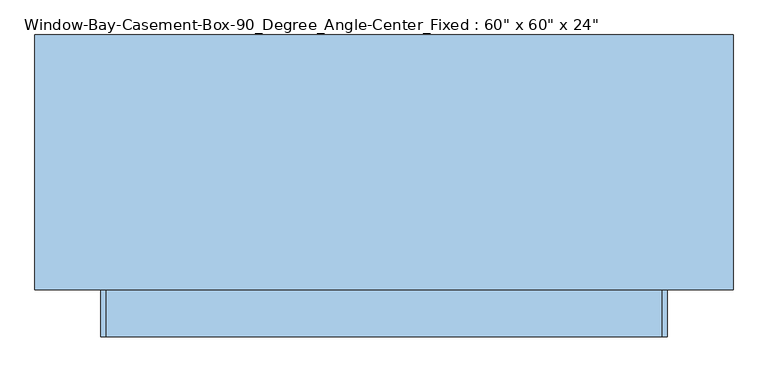
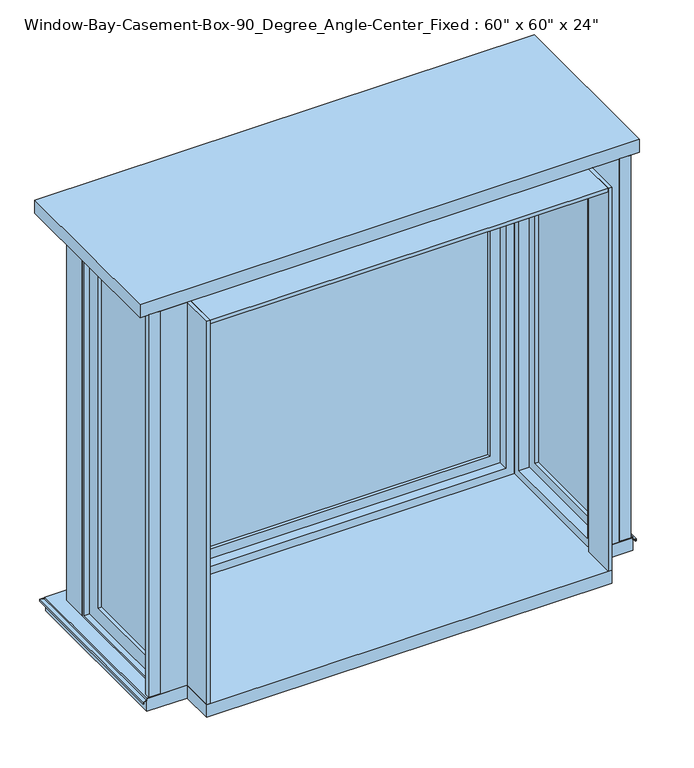
"""IFC4 building model written with IfcOpenShell, lengths in millimetres: window geometry."""

from ifc_helpers import new_model, si_unit, frame, origin, place, context, project, spatial, polyline, outline, extrude, faceted_brep, source, transform, mapped, element, save


def window_153fc52c(model_context):
    return source(origin(), model_context, "Body", "SolidModel", [
        extrude(outline(polyline([(-863.6, 63.5), (-908.05, 63.5), (-908.05, 82.55), (-863.6, 82.55), (-863.6, 63.5)])), frame((0.0, 0.0, 663.1486341), z_axis=(0.0, 0.0, 1.0), x_axis=(1.0, 0.0, 0.0)), (0.0, 0.0, 1.0), 1521.2513659),
        extrude(outline(polyline([(908.05, 63.5), (863.6, 63.5), (863.6, 82.55), (908.05, 82.55), (908.05, 63.5)])), frame((0.0, 0.0, 663.1486341), z_axis=(0.0, 0.0, 1.0), x_axis=(1.0, 0.0, 0.0)), (0.0, 0.0, 1.0), 1521.2513659),
        faceted_brep([(-914.4, 63.5, 653.0697935), (-914.4, 63.5, 660.4), (-863.6, 63.5, 660.4), (-863.6, 63.5, 663.1486341), (-915.797, 63.5, 663.1486341), (-915.797, 63.5, 654.4483503), (-928.497, 63.5, 652.2089977), (-928.497, 63.5, 643.2668038), (-924.5346, 63.5, 643.2668038), (-924.5346, 63.5, 644.7270038), (-926.8968, 63.5, 644.7270038), (-926.8968, 63.5, 650.8662705), (914.4, 63.5, 653.0697935), (926.8968, 63.5, 650.8662705), (926.8968, 63.5, 644.7270038), (924.5346, 63.5, 644.7270038), (924.5346, 63.5, 643.2668038), (928.497, 63.5, 643.2668038), (928.497, 63.5, 652.2089977), (915.797, 63.5, 654.4483503), (915.797, 63.5, 663.1486341), (863.6, 63.5, 663.1486341), (863.6, 63.5, 660.4), (914.4, 63.5, 660.4), (-914.4, 723.9, 653.0697935), (-914.4, 723.9, 660.4), (914.4, 723.9, 660.4), (863.6, 673.1, 660.4), (-863.6, 673.1, 660.4), (-863.6, 673.1, 663.1486341), (863.6, 673.1, 663.1486341), (915.797, 725.297, 663.1486341), (-915.797, 725.297, 663.1486341), (-915.797, 725.297, 654.4483503), (-928.497, 737.997, 652.2089977), (-928.497, 737.997, 643.2668038), (928.497, 737.997, 643.2668038), (924.5346, 734.0346, 643.2668038), (-924.5346, 734.0346, 643.2668038), (-924.5346, 734.0346, 644.7270038), (924.5346, 734.0346, 644.7270038), (926.8968, 736.3968, 644.7270038), (-926.8968, 736.3968, 644.7270038), (-926.8968, 736.3968, 650.8662705), (914.4, 723.9, 653.0697935), (915.797, 725.297, 654.4483503), (928.497, 737.997, 652.2089977), (926.8968, 736.3968, 650.8662705)], [[[0, 1, 2, 3, 4, 5, 6, 7, 8, 9, 10, 11]], [[12, 13, 14, 15, 16, 17, 18, 19, 20, 21, 22, 23]], [[1, 0, 24, 25]], [[2, 1, 25, 26, 23, 22, 27, 28]], [[3, 2, 28, 29]], [[4, 3, 29, 30, 21, 20, 31, 32]], [[5, 4, 32, 33]], [[6, 5, 33, 34]], [[7, 6, 34, 35]], [[8, 7, 35, 36, 17, 16, 37, 38]], [[9, 8, 38, 39]], [[10, 9, 39, 40, 15, 14, 41, 42]], [[11, 10, 42, 43]], [[0, 11, 43, 24]], [[25, 24, 44, 26]], [[29, 28, 27, 30]], [[33, 32, 31, 45]], [[34, 33, 45, 46]], [[35, 34, 46, 36]], [[39, 38, 37, 40]], [[43, 42, 41, 47]], [[24, 43, 47, 44]], [[26, 44, 12, 23]], [[30, 27, 22, 21]], [[45, 31, 20, 19]], [[46, 45, 19, 18]], [[36, 46, 18, 17]], [[40, 37, 16, 15]], [[47, 41, 14, 13]], [[44, 47, 13, 12]]]),
        extrude(outline(polyline([(914.4, 723.9), (914.4, 63.5), (762.0, 63.5), (762.0, -63.5), (-762.0, -63.5), (-762.0, 63.5), (-914.4, 63.5), (-914.4, 723.9), (914.4, 723.9)])), frame((0.0, 0.0, 609.6), z_axis=(0.0, 0.0, 1.0), x_axis=(1.0, 0.0, 0.0)), (0.0, 0.0, 1.0), 50.8),
        extrude(outline(polyline([(939.8, 749.3), (939.8, 63.5), (-939.8, 63.5), (-939.8, 749.3), (939.8, 749.3)])), frame((0.0, 0.0, 2184.4), z_axis=(0.0, 0.0, 1.0), x_axis=(1.0, 0.0, 0.0)), (0.0, 0.0, 1.0), 50.8),
        extrude(outline(polyline([(-762.0, 673.1), (-762.0, 571.5), (-863.6, 571.5), (-863.6, 673.1), (-762.0, 673.1)])), frame((0.0, 0.0, 660.4), z_axis=(0.0, 0.0, 1.0), x_axis=(1.0, 0.0, 0.0)), (0.0, 0.0, 1.0), 1524.0),
        extrude(outline(polyline([(863.6, 673.1), (863.6, 571.5), (762.0, 571.5), (762.0, 673.1), (863.6, 673.1)])), frame((0.0, 0.0, 660.4), z_axis=(0.0, 0.0, 1.0), x_axis=(1.0, 0.0, 0.0)), (0.0, 0.0, 1.0), 1524.0),
        faceted_brep([(749.3, 609.6, 673.1), (749.3, 673.1, 673.1), (-749.3, 673.1, 673.1), (-749.3, 609.6, 673.1), (730.25, 571.5, 692.15), (730.25, 609.6, 692.15), (-730.25, 609.6, 692.15), (-730.25, 571.5, 692.15), (762.0, 673.1, 660.4), (762.0, 571.5, 660.4), (-762.0, 571.5, 660.4), (-762.0, 673.1, 660.4), (-749.3, 673.1, 2171.7), (-749.3, 609.6, 2171.7), (-730.25, 609.6, 2152.65), (-730.25, 571.5, 2152.65), (-762.0, 571.5, 2184.4), (-762.0, 673.1, 2184.4), (749.3, 673.1, 2171.7), (749.3, 609.6, 2171.7), (730.25, 609.6, 2152.65), (730.25, 571.5, 2152.65), (762.0, 571.5, 2184.4), (762.0, 673.1, 2184.4)], [[[0, 1, 2, 3]], [[4, 5, 6, 7]], [[8, 9, 10, 11]], [[3, 2, 12, 13]], [[7, 6, 14, 15]], [[11, 10, 16, 17]], [[13, 12, 18, 19]], [[15, 14, 20, 21]], [[17, 16, 22, 23]], [[11, 17, 23, 8], [1, 18, 12, 2]], [[19, 18, 1, 0]], [[3, 13, 19, 0], [5, 20, 14, 6]], [[21, 20, 5, 4]], [[9, 22, 16, 10], [7, 15, 21, 4]], [[23, 22, 9, 8]]]),
        extrude(outline(polyline([(2171.7, -749.3), (673.1, -749.3), (673.1, 749.3), (2171.7, 749.3), (2171.7, -749.3)]), holes=[polyline([(2114.55, 692.15), (730.25, 692.15), (730.25, -692.15), (2114.55, -692.15), (2114.55, 692.15)])]), frame((0.0, 609.6, 0.0), z_axis=(0.0, 1.0, 0.0), x_axis=(0.0, 0.0, 1.0)), (0.0, 0.0, 1.0), 44.45),
        faceted_brep([(-762.0, 95.25, 2152.65), (-800.1, 95.25, 2152.65), (-800.1, 539.75, 2152.65), (-762.0, 539.75, 2152.65), (-863.6, 63.5, 2184.4), (-762.0, 63.5, 2184.4), (-762.0, 571.5, 2184.4), (-863.6, 571.5, 2184.4), (-800.1, 76.2, 2171.7), (-863.6, 76.2, 2171.7), (-863.6, 558.8, 2171.7), (-800.1, 558.8, 2171.7), (-800.1, 539.75, 692.15), (-762.0, 539.75, 692.15), (-762.0, 571.5, 660.4), (-863.6, 571.5, 660.4), (-863.6, 558.8, 673.1), (-800.1, 558.8, 673.1), (-800.1, 95.25, 692.15), (-762.0, 95.25, 692.15), (-762.0, 63.5, 660.4), (-863.6, 63.5, 660.4), (-863.6, 76.2, 673.1), (-800.1, 76.2, 673.1)], [[[0, 1, 2, 3]], [[4, 5, 6, 7]], [[8, 9, 10, 11]], [[3, 2, 12, 13]], [[7, 6, 14, 15]], [[11, 10, 16, 17]], [[13, 12, 18, 19]], [[15, 14, 20, 21]], [[17, 16, 22, 23]], [[11, 17, 23, 8], [1, 18, 12, 2]], [[19, 18, 1, 0]], [[5, 20, 14, 6], [3, 13, 19, 0]], [[21, 20, 5, 4]], [[7, 15, 21, 4], [9, 22, 16, 10]], [[23, 22, 9, 8]]]),
        extrude(outline(polyline([(558.8, 2171.7), (558.8, 673.1), (76.2, 673.1), (76.2, 2171.7), (558.8, 2171.7)]), holes=[polyline([(133.35, 2114.55), (133.35, 730.25), (501.65, 730.25), (501.65, 2114.55), (133.35, 2114.55)])]), frame((-844.55, 0.0, 0.0), z_axis=(1.0, 0.0, 0.0), x_axis=(0.0, 1.0, 0.0)), (0.0, 0.0, 1.0), 44.45),
        faceted_brep([(800.1, 95.25, 2152.65), (762.0, 95.25, 2152.65), (762.0, 539.75, 2152.65), (800.1, 539.75, 2152.65), (863.6, 76.2, 2171.7), (800.1, 76.2, 2171.7), (800.1, 558.8, 2171.7), (863.6, 558.8, 2171.7), (762.0, 63.5, 2184.4), (863.6, 63.5, 2184.4), (863.6, 571.5, 2184.4), (762.0, 571.5, 2184.4), (762.0, 539.75, 692.15), (800.1, 539.75, 692.15), (800.1, 558.8, 673.1), (863.6, 558.8, 673.1), (863.6, 571.5, 660.4), (762.0, 571.5, 660.4), (762.0, 95.25, 692.15), (800.1, 95.25, 692.15), (800.1, 76.2, 673.1), (863.6, 76.2, 673.1), (863.6, 63.5, 660.4), (762.0, 63.5, 660.4)], [[[0, 1, 2, 3]], [[4, 5, 6, 7]], [[8, 9, 10, 11]], [[3, 2, 12, 13]], [[7, 6, 14, 15]], [[11, 10, 16, 17]], [[13, 12, 18, 19]], [[15, 14, 20, 21]], [[17, 16, 22, 23]], [[11, 17, 23, 8], [1, 18, 12, 2]], [[19, 18, 1, 0]], [[5, 20, 14, 6], [3, 13, 19, 0]], [[21, 20, 5, 4]], [[9, 22, 16, 10], [7, 15, 21, 4]], [[23, 22, 9, 8]]]),
        extrude(outline(polyline([(558.8, 2171.7), (558.8, 673.1), (76.2, 673.1), (76.2, 2171.7), (558.8, 2171.7)]), holes=[polyline([(133.35, 2114.55), (133.35, 730.25), (501.65, 730.25), (501.65, 2114.55), (133.35, 2114.55)])]), frame((800.1, 0.0, 0.0), z_axis=(1.0, 0.0, 0.0), x_axis=(0.0, 1.0, 0.0)), (0.0, 0.0, 1.0), 44.45),
        extrude(outline(polyline([(692.15, 641.35), (692.15, 635.0), (-692.15, 635.0), (-692.15, 641.35), (692.15, 641.35)])), frame((0.0, 0.0, 730.25), z_axis=(0.0, 0.0, 1.0), x_axis=(1.0, 0.0, 0.0)), (0.0, 0.0, 1.0), 1384.3),
        extrude(outline(polyline([(692.15, 628.65), (692.15, 622.3), (-692.15, 622.3), (-692.15, 628.65), (692.15, 628.65)])), frame((0.0, 0.0, 730.25), z_axis=(0.0, 0.0, 1.0), x_axis=(1.0, 0.0, 0.0)), (0.0, 0.0, 1.0), 1384.3),
        extrude(outline(polyline([(-825.5, 501.65), (-825.5, 133.35), (-831.85, 133.35), (-831.85, 501.65), (-825.5, 501.65)])), frame((0.0, 0.0, 730.25), z_axis=(0.0, 0.0, 1.0), x_axis=(1.0, 0.0, 0.0)), (0.0, 0.0, 1.0), 1384.3),
        extrude(outline(polyline([(-812.8, 501.65), (-812.8, 133.35), (-819.15, 133.35), (-819.15, 501.65), (-812.8, 501.65)])), frame((0.0, 0.0, 730.25), z_axis=(0.0, 0.0, 1.0), x_axis=(1.0, 0.0, 0.0)), (0.0, 0.0, 1.0), 1384.3),
        extrude(outline(polyline([(831.85, 501.65), (831.85, 133.35), (825.5, 133.35), (825.5, 501.65), (831.85, 501.65)])), frame((0.0, 0.0, 730.25), z_axis=(0.0, 0.0, 1.0), x_axis=(1.0, 0.0, 0.0)), (0.0, 0.0, 1.0), 1384.3),
        extrude(outline(polyline([(819.15, 501.65), (819.15, 133.35), (812.8, 133.35), (812.8, 501.65), (819.15, 501.65)])), frame((0.0, 0.0, 730.25), z_axis=(0.0, 0.0, 1.0), x_axis=(1.0, 0.0, 0.0)), (0.0, 0.0, 1.0), 1384.3),
        faceted_brep([(863.6, 76.2, 2171.7), (800.1, 76.2, 2171.7), (800.1, 558.8, 2171.7), (863.6, 558.8, 2171.7), (762.0, 63.5, 2184.4), (863.6, 63.5, 2184.4), (863.6, 571.5, 2184.4), (762.0, 571.5, 2184.4), (800.1, 95.25, 2152.65), (762.0, 95.25, 2152.65), (762.0, 539.75, 2152.65), (800.1, 539.75, 2152.65), (800.1, 558.8, 673.1), (863.6, 558.8, 673.1), (863.6, 571.5, 660.4), (762.0, 571.5, 660.4), (762.0, 539.75, 692.15), (800.1, 539.75, 692.15), (800.1, 76.2, 673.1), (863.6, 76.2, 673.1), (863.6, 63.5, 660.4), (762.0, 63.5, 660.4), (762.0, 95.25, 692.15), (800.1, 95.25, 692.15)], [[[0, 1, 2, 3]], [[4, 5, 6, 7]], [[8, 9, 10, 11]], [[3, 2, 12, 13]], [[7, 6, 14, 15]], [[11, 10, 16, 17]], [[13, 12, 18, 19]], [[15, 14, 20, 21]], [[17, 16, 22, 23]], [[1, 18, 12, 2], [11, 17, 23, 8]], [[19, 18, 1, 0]], [[5, 20, 14, 6], [3, 13, 19, 0]], [[21, 20, 5, 4]], [[7, 15, 21, 4], [9, 22, 16, 10]], [[23, 22, 9, 8]]]),
        extrude(outline(polyline([(-749.3, 63.5), (-749.3, -63.5), (-762.0, -63.5), (-762.0, 63.5), (-749.3, 63.5)])), frame((0.0, 0.0, 660.4), z_axis=(0.0, 0.0, 1.0), x_axis=(1.0, 0.0, 0.0)), (0.0, 0.0, 1.0), 1524.0),
        extrude(outline(polyline([(749.3, 63.5), (762.0, 63.5), (762.0, -63.5), (749.3, -63.5), (749.3, 63.5)])), frame((0.0, 0.0, 660.4), z_axis=(0.0, 0.0, 1.0), x_axis=(1.0, 0.0, 0.0)), (0.0, 0.0, 1.0), 1524.0),
        extrude(outline(polyline([(749.3, -63.5), (-749.3, -63.5), (-749.3, 571.5), (749.3, 571.5), (749.3, -63.5)])), frame((0.0, 0.0, 2171.7), z_axis=(0.0, 0.0, 1.0), x_axis=(1.0, 0.0, 0.0)), (0.0, 0.0, 1.0), 12.7),
    ])


if __name__ == "__main__":
    model = new_model("IFC4")
    model_context = context("Model", 3, world=origin())
    ifc_project = project(units=[si_unit("LENGTHUNIT", "METRE", prefix="MILLI")], contexts=[model_context])
    site = spatial("IfcSite", under=ifc_project)
    building = spatial("IfcBuilding", under=site)
    placement = place(None, origin())
    window_shape = window_153fc52c(model_context)
    element("IfcWindow", 1, ObjectType="Window-Bay-Casement-Box-90_Degree_Angle-Center_Fixed : 60\" x 60\" x 24\"", at=placement, inside=building, context=model_context, shape_type="MappedRepresentation", body=[
        mapped(window_shape, transform((0.0, 0.0, 0.0), x_axis=(1.0, 0.0, 0.0), y_axis=(0.0, 1.0, 0.0), z_axis=(0.0, 0.0, 1.0))),
    ])
    save(model, "model.ifc")

# Revit data of these elements
# Type "Window-Bay-Casement-Box-90_Degree_Angle-Center_Fixed : 60\" x 60\" x 24\""
#   Type Mark = "18"
#   Fire Rating = "0.5h"
#   Assembly Code = "B2020100"
#   Analytic Construction = "1/8 in Pilkington single glazing"
#   Width = 5' - 0"
#   Wall Thickness [instance default] = 0' - 6"
#   Visual Light Transmittance = 0.9
#   Trim Width = 5' - 8"
#   Trim Height = 5' - 0"
#   Thermal Resistance (R) = 1.5394 (h·ft²·°F)/BTU
#   Solar Heat Gain Coefficient = 0.86
#   Rough Width = 5' - 0 1/2"
#   Rough Height = 5' - 0 1/2"
#   Height 1 = 5' - 2"
#   Height = 5' - 0"
#   Heat Transfer Coefficient (U) = 0.6496 BTU/(h·ft²·°F)
#   Depth = 2' - 0"
#   Default Sill Height = 2' - 0"
#   Side Muntin Visibility = yes
#   Center Muntin Visibility = yes
#   Interior Trim Visibility [instance default] = yes
#   Exterior Trim Visibility [instance default] = yes
#   Side Muntin Pattern = Muntin Pattern_2x2 : Muntin Pattern_2x2
#   Center Muntin Pattern = Muntin Pattern_2x2 : Muntin Pattern_2x2
#   Interior Trim Material = Wood - Stained
#   Exterior Trim Material = Clad - White
#   Exterior Trim = element 393412
#   Interior Trim = Trim-Window-Interior-Flat : Picture Frame
#   Interior Frame Material = Wood - Stained
#   Glass Panel Material = Glass
#   Exterior Frame Material = Clad - White
#   Wall Closure = (empty or 0)
# Element 1 (IfcWindow, "Window-Bay-Casement-Box-90_Degree_Angle-Center_Fixed : 60\" x 60\" x 24\"")
#   Wall Thickness = 0' - 5"
#   Materials on its faces: "Clad - White", "Wood - Stained", "Glass"
# Materials
#   "Wood - Stained": class "Wood", colour RGB 224 178 126, transparency 0, Cost = 0
#   "Clad - White": class "Wood", colour RGB 242 242 238, transparency 0, Cost = 0
#   "Glass": class "Glass", colour RGB 0 128 192, transparency 0.75, Description = "Soda Lime Glass", Cost = 0
